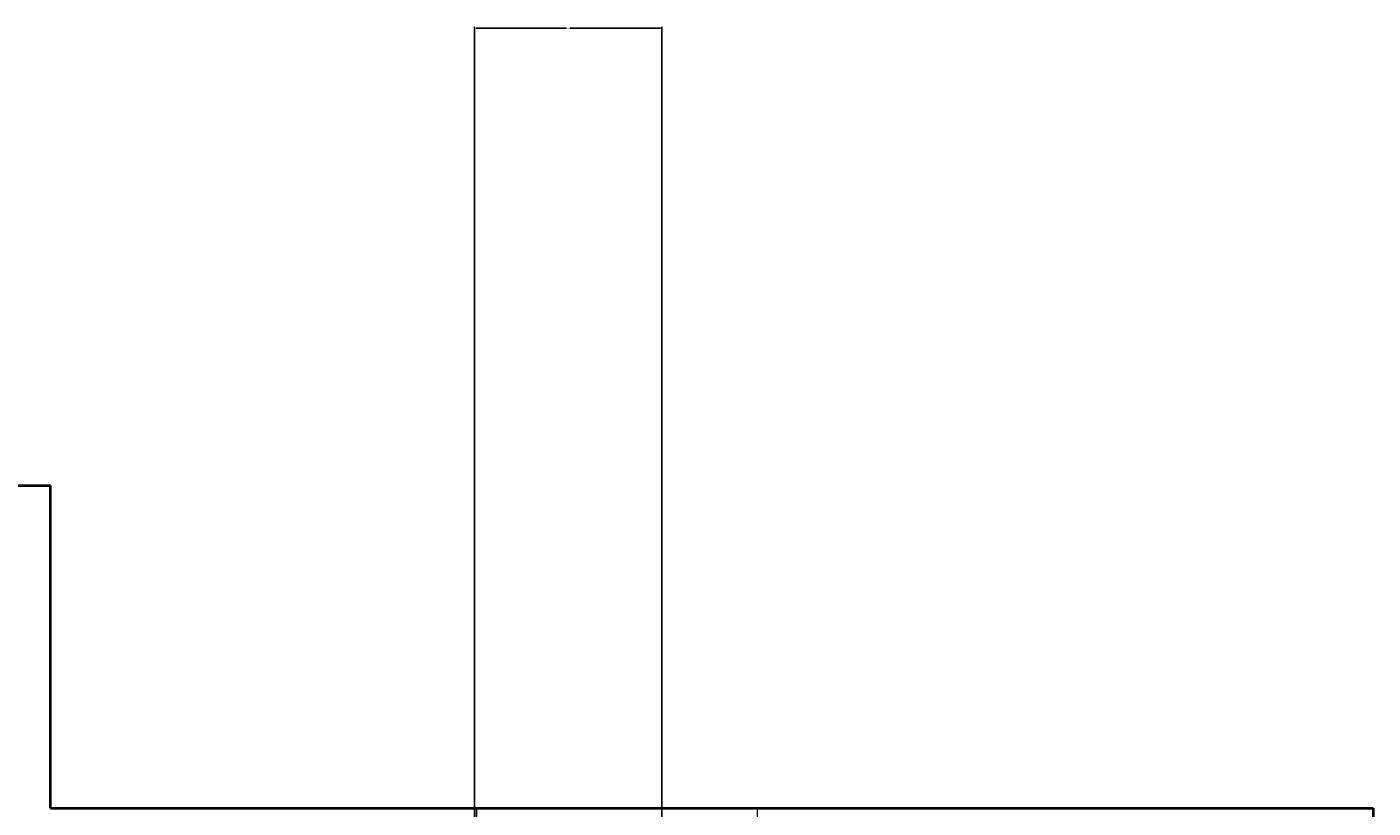
# Model space of a CAD drawing. Units: inches. Extents: x -46 to 1145, y -527 to 760.
# Tile 53 of 57: x 337 to 509, y 660 to 760. Entities that reach past the tile are written whole.
import ezdxf

# ---------------------------------------------------------------- set-up
doc = ezdxf.new("R2010")
doc.units = ezdxf.units.IN
doc.header["$MEASUREMENT"] = 0
for name, color, linetype, lineweight in [('A-ANNO-DIMS', 2, 'Continuous', 18), ('WALLS', 4, 'Continuous', 40), ('WINDOWS', 240, 'Continuous', 20)]:
    doc.layers.add(name, color=color, linetype=linetype, lineweight=lineweight)
doc.styles.get("Standard").update_dxf_attribs({"font": 'arial.ttf'})
doc.dimstyles.get("Standard").update_dxf_attribs({"dimtxt": 0.18, "dimasz": 0.18, "dimexe": 0.18, "dimexo": 0.0625, "dimgap": 0.09, "dimtad": 0, "dimtih": 1, "dimtoh": 1, "dimdec": 0, "dimzin": 0, "dimdsep": 46, "dimlunit": 3, "dimtxsty": 'Standard', "dimcen": 0.09, "dimadec": 0, "dimazin": 0, "dimtfac": 1, "dimtdec": 0, "dimtofl": 0, "dimtmove": 0, "dimatfit": 3, "dimfxl": 1, "dimtolj": 1, "dimtzin": 0, "dimarcsym": 0})

# ---------------------------------------------------------------- blocks, each defined once
blk = doc.blocks.new('WINDOW-36IN')
for p, q in [((0, 4.5), (0, 9)), ((0, 9), (0, 0)), ((36, 9), (36, 0)), ((0, 5.23), (36, 5.23)), ((0, 4.5), (36, 4.5))]:
    blk.add_line(p, q)
blk = doc.blocks.new('*D699')
at = {"layer": 'A-ANNO-DIMS', "color": 0, "lineweight": -2, "transparency": 16777216}
for p, q in [((393.93, 530.58), (393.93, 759.67)), ((394.11, 759.49), (405.71, 759.49)), ((417.75, 759.49), (406.15, 759.49)), ((417.93, 530.58), (417.93, 759.67))]:
    blk.add_line(p, q, dxfattribs=at)
at = {"layer": 'A-ANNO-DIMS', "color": 0, "transparency": 16777216}
for points in [[(394.11, 759.52), (394.11, 759.46), (393.93, 759.49)], [(417.75, 759.52), (417.75, 759.46), (417.93, 759.49)]]:
    blk.add_solid(points, dxfattribs=at)
at = {"layer": 'Defpoints', "color": 0, "transparency": 16777216}
for p in [(417.93, 759.49), (393.93, 530.52), (417.93, 530.52)]:
    blk.add_point(p, dxfattribs=at)
at = {"layer": 'A-ANNO-DIMS', "color": 0, "transparency": 16777216, "insert": (405.93, 759.49), "char_height": 0.18, "attachment_point": 5}
blk.add_mtext('\\A1;24', dxfattribs=at)

msp = doc.modelspace()

# ---------------------------------------------------------------- linework, layer by layer
at = {"layer": 'WALLS'}
for p, q in [((189.5637, 700.8886), (339.5637, 700.8886)), ((339.5637, 659.5176), (339.5637, 700.8886)), ((339.5637, 659.5176), (509.0637, 659.5176)), ((509.0637, 659.5176), (509.0637, 221.5176))]:
    msp.add_line(p, q, dxfattribs=at)

# ---------------------------------------------------------------- block references
at = {"layer": 'WINDOWS'}
msp.add_blockref('WINDOW-36IN', (394.1543, 650.518), dxfattribs=at)

# ---------------------------------------------------------------- dimensions: what is measured, and where the dimension line sits
at = {"layer": 'A-ANNO-DIMS'}
dim = msp.add_linear_dim(base=(417.9282, 759.4886), p1=(393.9282, 530.5176), p2=(417.9282, 530.5176), dimstyle='Standard', override={"dimdec": 0, "dimlfac": 1, "dimrnd": 0, "dimzin": 0, "dimdsep": 46, "dimlunit": 2}, dxfattribs=at)
dim.commit()
dim.dimension.update_dxf_attribs({"geometry": '*D699', "text_midpoint": (405.9282, 759.4886)})

doc.saveas('drawing.dxf')
